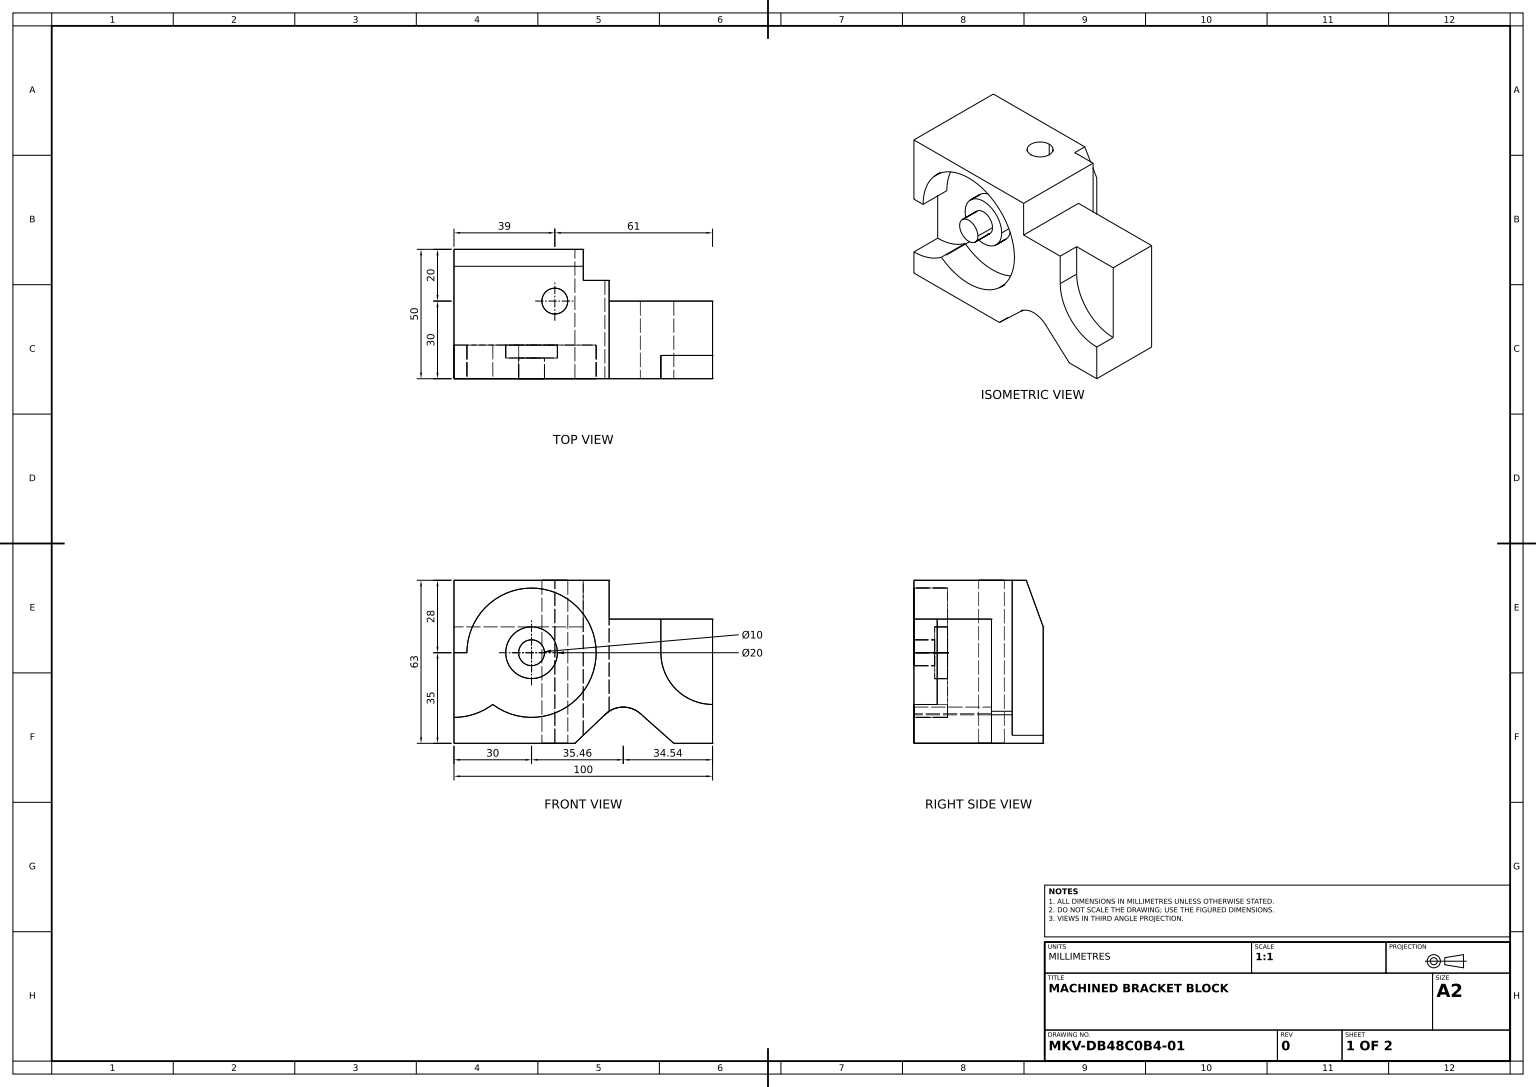
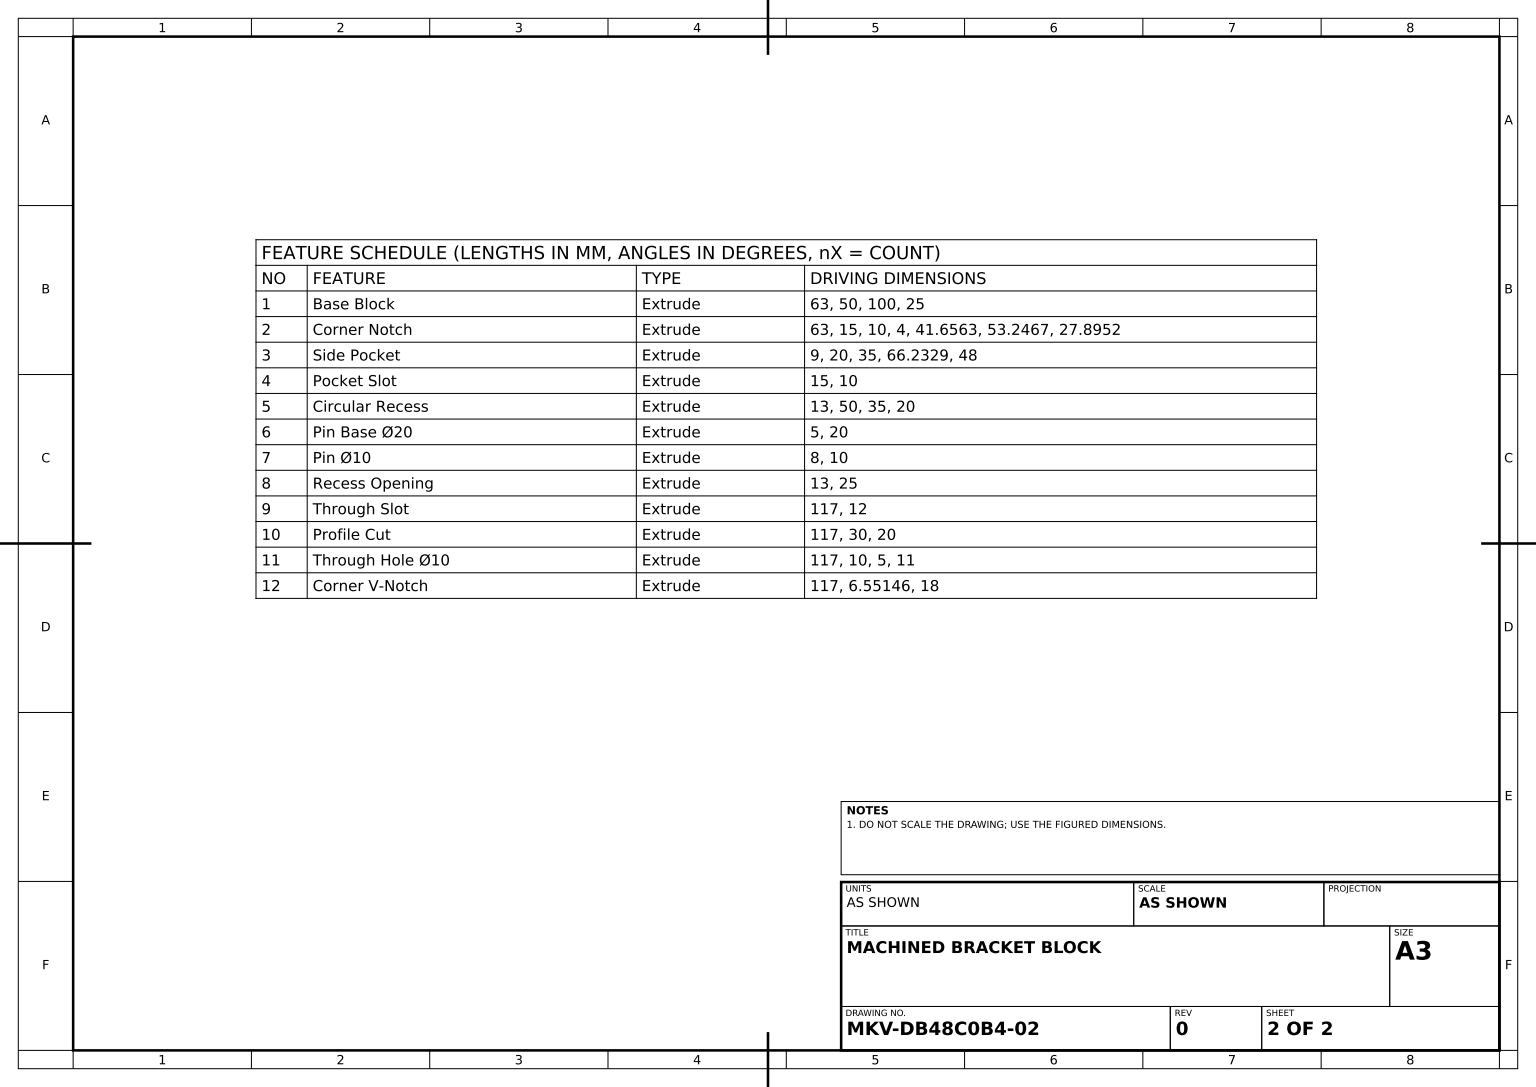
from build123d import *

# Parameters (mm, degrees)
BASE_BLOCK_DEPTH         = 63
CORNER_NOTCH_DEPTH       = 63
SIDE_POCKET_SKETCH_W     = 20
SIDE_POCKET_SKETCH_H     = 3.232862168
SIDE_POCKET_DEPTH        = 9
POCKET_SLOT_SKETCH_W     = 40
POCKET_SLOT_SKETCH_H     = 50
POCKET_SLOT_DEPTH        = 15
CIRCULAR_RECESS_SKETCH_R = 25
CIRCULAR_RECESS_DEPTH    = 13
PIN_BASE_20_SKETCH_R     = 10
PIN_BASE_20_DEPTH        = 5
PIN_10_SKETCH_R          = 5
PIN_10_DEPTH             = 8
RECESS_OPENING_DEPTH     = 13
THROUGH_SLOT_SKETCH_W    = 10
THROUGH_SLOT_SKETCH_H    = 12
THROUGH_SLOT_DEPTH       = 117
PROFILE_CUT_DEPTH        = 117
THROUGH_HOLE_10_SKETCH_R = 5
THROUGH_HOLE_10_DEPTH    = 117
CORNER_V_NOTCH_DEPTH     = 117


with BuildPart() as part:
    # Base Block Sketch → Base Block (new body)
    with BuildSketch(Plane(origin=(0, 0, 0), x_dir=(1, 0, 0), z_dir=(0, 1, 0))):
        Polygon((50, 0), (50, 25), (-50, 25), (-50, -25), (50, -25), align=None)
    extrude(amount=BASE_BLOCK_DEPTH)

    # Corner Notch Sketch → Corner Notch (cut)
    with BuildSketch(Plane.XY.offset(25)):
        with BuildLine():
            Line((35, 0), (22.104816934, 11.471476847))
            ThreePointArc((22.104816934, 11.471476847), (15.135621173, 13.994794618), (8.343659927, 11.027289849))
            Line((8.343659927, 11.027289849), (-3.246679913, 0))
            Line((-3.246679913, 0), (35, 0))
        make_face()
    extrude(amount=-CORNER_NOTCH_DEPTH, mode=Mode.SUBTRACT)

    # Side Pocket Sketch → Side Pocket (cut)
    with BuildSketch(Plane.XY.offset(25)):
        with BuildLine():
            ThreePointArc((30, 35), (35.857864376, 20.857864376), (50, 15))
            Line((50, 15), (50, 35))
            Line((50, 35), (50, 63))
            Line((50, 63), (30, 63))
            Line((30, 63), (30, 48))
            Line((30, 48), (30, 35))
        make_face()
        with Locations((40, 64.616431084)):
            Rectangle(SIDE_POCKET_SKETCH_W, SIDE_POCKET_SKETCH_H)
    extrude(amount=-SIDE_POCKET_DEPTH, mode=Mode.SUBTRACT)

    # Pocket Slot Sketch → Pocket Slot (cut)
    with BuildSketch(Plane(origin=(0, 63, 0), x_dir=(1, 0, 0), z_dir=(0, 1, 0))):
        with Locations((30, 0)):
            Rectangle(POCKET_SLOT_SKETCH_W, POCKET_SLOT_SKETCH_H)
    extrude(amount=-POCKET_SLOT_DEPTH, mode=Mode.SUBTRACT)

    # Circular Recess Sketch → Circular Recess (cut)
    with BuildSketch(Plane.XY.offset(25)):
        with Locations((-20, 35)):
            Circle(CIRCULAR_RECESS_SKETCH_R)
    extrude(amount=-CIRCULAR_RECESS_DEPTH, mode=Mode.SUBTRACT)

    # Pin Base Ø20 Sketch → Pin Base Ø20 (add)
    with BuildSketch(Plane.XY.offset(12)):
        with Locations((-20, 35)):
            Circle(PIN_BASE_20_SKETCH_R)
    extrude(amount=PIN_BASE_20_DEPTH)

    # Pin Ø10 Sketch → Pin Ø10 (add)
    with BuildSketch(Plane.XY.offset(17)):
        with Locations((-20, 35)):
            Circle(PIN_10_SKETCH_R)
    extrude(amount=PIN_10_DEPTH)

    # Recess Opening Sketch → Recess Opening (cut)
    with BuildSketch(Plane.XY.offset(25)):
        with BuildLine():
            Line((-45, 35), (-50, 35))
            Line((-50, 35), (-50, 10))
            ThreePointArc((-50, 10), (-42.09430585, 11.282917549), (-35, 15))
            ThreePointArc((-35, 15), (-42.360679775, 23.819660113), (-45, 35))
        make_face()
    extrude(amount=-RECESS_OPENING_DEPTH, mode=Mode.SUBTRACT)

    # Through Slot Sketch → Through Slot (cut)
    with BuildSketch(Plane(origin=(0, 63, 0), x_dir=(1, 0, 0), z_dir=(0, 1, 0))):
        with Locations((5, 19)):
            Rectangle(THROUGH_SLOT_SKETCH_W, THROUGH_SLOT_SKETCH_H)
    extrude(amount=-THROUGH_SLOT_DEPTH, mode=Mode.SUBTRACT)

    # Profile Cut Sketch → Profile Cut (cut)
    with BuildSketch(Plane(origin=(0, 48, 0), x_dir=(1, 0, 0), z_dir=(0, 1, 0))):
        Polygon((20, 5), (50, 5), (50, 25), (10, 25), (10, 5), align=None)
    extrude(amount=-PROFILE_CUT_DEPTH, mode=Mode.SUBTRACT)

    # Through Hole Ø10 Sketch → Through Hole Ø10 (cut)
    with BuildSketch(Plane(origin=(0, 63, 0), x_dir=(1, 0, 0), z_dir=(0, 1, 0))):
        with Locations(Location((-11, 5, 0), (0, 0, 270))):
            Circle(THROUGH_HOLE_10_SKETCH_R)
    extrude(amount=-THROUGH_HOLE_10_DEPTH, mode=Mode.SUBTRACT)

    # Corner V-Notch Sketch → Corner V-Notch (cut)
    with BuildSketch(Plane.ZY.offset(50)):
        Polygon((-25, 63), (-25, 45), (-18.448535783, 63), align=None)
    extrude(amount=-CORNER_V_NOTCH_DEPTH, mode=Mode.SUBTRACT)


solid = part.part
